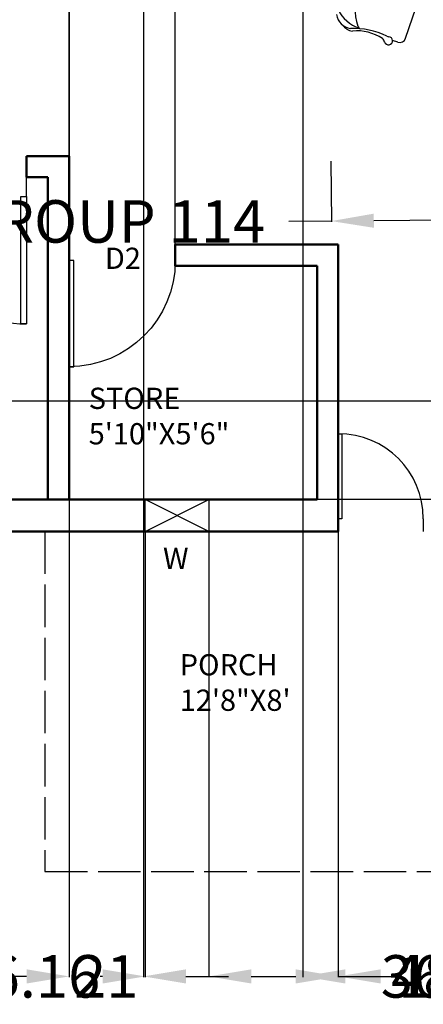
# Model space of a CAD drawing. Units: inches. Extents: x -77 to 516, y -119 to 536.
# Tile 2 of 11: x 150 to 264, y -119 to 159. Entities that reach past the tile are written whole.
import ezdxf

# ---------------------------------------------------------------- set-up
doc = ezdxf.new("R2010")
doc.units = ezdxf.units.IN
doc.header["$MEASUREMENT"] = 0
doc.linetypes.add('ACAD_ISO02W100', pattern=[15, 12, -3])
for name, color, linetype, lineweight in [('A-ANNO-DIMS', 2, 'Continuous', 18), ('A-AREA-IDEN', 170, 'Continuous', 25), ('A-FLOR-PRCH', 40, 'ACAD_ISO02W100', 25), ('doors', 6, 'Continuous', 25), ('furniture', 119, 'Continuous', 18), ('text', 170, 'Continuous', 18), ('walls', 40, 'Continuous', 50), ('windows', 1, 'Continuous', 25)]:
    doc.layers.add(name, color=color, linetype=linetype, lineweight=lineweight)
doc.layers.add('FUR', color=42, linetype='Continuous')
doc.styles.get("Standard").update_dxf_attribs({"font": 'arial.ttf'})
doc.dimstyles.get("Standard").update_dxf_attribs({"dimtxt": 12, "dimasz": 12, "dimexe": 0.18, "dimexo": 0.0625, "dimgap": 0.09, "dimtad": 0, "dimtih": 1, "dimtoh": 1, "dimdec": 1, "dimzin": 0, "dimdsep": 46, "dimlunit": 4, "dimtxsty": 'Standard', "dimcen": 0.09, "dimadec": 0, "dimazin": 0, "dimtfac": 1, "dimtdec": 1, "dimtofl": 0, "dimtmove": 0, "dimatfit": 3, "dimfxl": 1, "dimtolj": 1, "dimtzin": 0, "dimarcsym": 0})

# ---------------------------------------------------------------- blocks, each defined once
blk = doc.blocks.new('*U2')
for p, q in [((0, 0), (0, -6)), ((40, 0), (40, -6))]:
    blk.add_line(p, q)
blk.add_lwpolyline([(0, 0), (0, 40), (1.75, 40), (1.75, 0)], close=True)
blk.add_arc((0, 0), 40, 0, 90)
blk = doc.blocks.new('A$C44A37715')
at = {"layer": 'FUR'}
for p, q in [((3.646, 2.261), (3.416, 1.609)), ((3.734, 2.304), (3.792, 2.283))]:
    blk.add_line(p, q, dxfattribs=at)
for centre, radius, start, end in [((3.837, 2.287), 0.0455, 16.8807, 266.7473), ((3.711, 2.238), 0.0691, 70.5477, 160.5477), ((3.831, 2.187), 0.0553, 63.6571, 86.7473), ((4.239, 3.009), 0.863, 243.6571, 271.4769), ((3.936, 2.308), 0.0553, 187.894, 235.9057), ((4.195, 2.692), 0.519, 235.9057, 274.894), ((3.567, 1.923), 0.642, 303.2315, 17.8639), ((4.125, 2.102), 0.0553, 17.8639, 64.7798), ((4.037, 1.769), 0.394, 24.5429, 71.319), ((4.219, 2.021), 0.155, 33.6596, 82.2991), ((4.228, 1.96), 0.19, 8.9926, 80.0637)]:
    blk.add_arc(centre, radius, start, end, dxfattribs=at)
blk = doc.blocks.new('WIN-18IN')
for p, q in [((18, 0), (0, 9)), ((0, 0), (18, 9))]:
    blk.add_line(p, q)
blk.add_lwpolyline([(0, 9), (18, 9), (18, 0), (0, 0)], close=True)
blk = doc.blocks.new('*D30')
at = {"layer": 'A-ANNO-DIMS', "color": 0, "lineweight": -2, "transparency": 16777216}
for p, q in [((351.13, 120.17), (351.28, 103.03)), ((237.64, 119.18), (237.79, 102.04)), ((339.28, 103.1), (249.78, 102.32)), ((237.78, 102.22), (225.78, 102.12))]:
    blk.add_line(p, q, dxfattribs=at)
at = {"layer": 'A-ANNO-DIMS', "color": 0, "transparency": 16777216}
for points in [[(249.77, 104.32), (249.8, 100.32), (237.78, 102.22)], [(339.27, 105.1), (339.3, 101.1), (351.28, 103.21)]]:
    blk.add_solid(points, dxfattribs=at)
at = {"layer": 'Defpoints', "color": 0, "transparency": 16777216}
for p in [(351.13, 120.23), (237.64, 119.24), (237.78, 102.22)]:
    blk.add_point(p, dxfattribs=at)
at = {"layer": 'A-ANNO-DIMS', "color": 0, "transparency": 16777216, "insert": (140.3, 102.12), "char_height": 12, "attachment_point": 5}
blk.add_mtext('\\A1;SEATING GROUP 114', dxfattribs=at)
blk = doc.blocks.new('*D40')
at = {"layer": 'A-ANNO-DIMS', "color": 0, "lineweight": -2, "transparency": 16777216}
for p, q in [((163.750061, 485.5259), (163.750061, -111.2416)), ((184.750061, 485.5259), (184.750061, -111.2416)), ((151.750061, -111.0616), (139.750061, -111.0616)), ((196.750061, -111.0616), (208.750061, -111.0616))]:
    blk.add_line(p, q, dxfattribs=at)
at = {"layer": 'A-ANNO-DIMS', "color": 0, "transparency": 16777216}
for points in [[(151.750061, -109.0616), (151.750061, -113.0616), (163.750061, -111.0616)], [(196.750061, -109.0616), (196.750061, -113.0616), (184.750061, -111.0616)]]:
    blk.add_solid(points, dxfattribs=at)
at = {"layer": 'Defpoints', "color": 0, "transparency": 16777216}
for p in [(163.750061, 485.5884), (184.750061, 485.5884), (184.750061, -111.0616)]:
    blk.add_point(p, dxfattribs=at)
at = {"layer": 'A-ANNO-DIMS', "color": 0, "transparency": 16777216, "insert": (174.250061, -111.0616), "char_height": 12, "attachment_point": 5}
blk.add_mtext('\\A1;21', dxfattribs=at)
blk = doc.blocks.new('*D41')
at = {"layer": 'A-ANNO-DIMS', "color": 0, "lineweight": -2, "transparency": 16777216}
for p, q in [((229.75, 485.53), (229.75, -111.24)), ((333.59, 485.53), (333.59, -111.24)), ((241.75, -111.06), (257.26, -111.06)), ((321.59, -111.06), (306.08, -111.06))]:
    blk.add_line(p, q, dxfattribs=at)
at = {"layer": 'A-ANNO-DIMS', "color": 0, "transparency": 16777216}
for points in [[(241.75, -109.06), (241.75, -113.06), (229.75, -111.06)], [(321.59, -109.06), (321.59, -113.06), (333.59, -111.06)]]:
    blk.add_solid(points, dxfattribs=at)
at = {"layer": 'Defpoints', "color": 0, "transparency": 16777216}
for p in [(229.75, 485.59), (333.59, 485.59), (333.59, -111.06)]:
    blk.add_point(p, dxfattribs=at)
at = {"layer": 'A-ANNO-DIMS', "color": 0, "transparency": 16777216, "insert": (281.67, -111.06), "char_height": 12, "attachment_point": 5}
blk.add_mtext('\\A1;103.84', dxfattribs=at)
blk = doc.blocks.new('*D45')
at = {"layer": 'A-ANNO-DIMS', "color": 0, "lineweight": -2, "transparency": 16777216}
for p, q in [((-15.9, 51.35), (-15.9, 63.35)), ((-15.9, 63.35), (-3.9, 63.35)), ((364.69, 51.35), (-16.08, 51.35)), ((-15.9, 35.59), (-15.9, 39.35)), ((364.69, 23.59), (-16.08, 23.59))]:
    blk.add_line(p, q, dxfattribs=at)
at = {"layer": 'A-ANNO-DIMS', "color": 0, "transparency": 16777216}
for points in [[(-17.9, 39.35), (-13.9, 39.35), (-15.9, 51.35)], [(-17.9, 35.59), (-13.9, 35.59), (-15.9, 23.59)]]:
    blk.add_solid(points, dxfattribs=at)
at = {"layer": 'Defpoints', "color": 0, "transparency": 16777216}
for p in [(-15.9, 51.35), (364.75, 51.35), (364.75, 23.59)]:
    blk.add_point(p, dxfattribs=at)
at = {"layer": 'A-ANNO-DIMS', "color": 0, "transparency": 16777216, "insert": (16.54, 63.35), "char_height": 12, "attachment_point": 5}
blk.add_mtext('\\A1;27.76', dxfattribs=at)
blk = doc.blocks.new('*D50')
at = {"layer": 'A-ANNO-DIMS', "color": 0, "lineweight": -2, "transparency": 16777216}
for p, q in [((119.05, 14.53), (119.05, -111.24)), ((185.2, 14.53), (185.2, -111.24)), ((131.05, -111.06), (131.76, -111.06)), ((173.2, -111.06), (172.49, -111.06))]:
    blk.add_line(p, q, dxfattribs=at)
at = {"layer": 'A-ANNO-DIMS', "color": 0, "transparency": 16777216}
for points in [[(131.05, -109.06), (131.05, -113.06), (119.05, -111.06)], [(173.2, -109.06), (173.2, -113.06), (185.2, -111.06)]]:
    blk.add_solid(points, dxfattribs=at)
at = {"layer": 'Defpoints', "color": 0, "transparency": 16777216}
for p in [(119.05, 14.59), (185.2, 14.59), (185.2, -111.06)]:
    blk.add_point(p, dxfattribs=at)
at = {"layer": 'A-ANNO-DIMS', "color": 0, "transparency": 16777216, "insert": (152.12, -111.06), "char_height": 12, "attachment_point": 5}
blk.add_mtext('\\A1;66.16', dxfattribs=at)
blk = doc.blocks.new('*D51')
at = {"layer": 'A-ANNO-DIMS', "color": 0, "lineweight": -2, "transparency": 16777216}
for p, q in [((203.2, 14.53), (203.2, -111.24)), ((239.75, 14.53), (239.75, -111.24)), ((215.2, -111.06), (227.75, -111.06)), ((239.75, -111.06), (251.75, -111.06))]:
    blk.add_line(p, q, dxfattribs=at)
at = {"layer": 'A-ANNO-DIMS', "color": 0, "transparency": 16777216}
for points in [[(215.2, -109.06), (215.2, -113.06), (203.2, -111.06)], [(227.75, -109.06), (227.75, -113.06), (239.75, -111.06)]]:
    blk.add_solid(points, dxfattribs=at)
at = {"layer": 'Defpoints', "color": 0, "transparency": 16777216}
for p in [(203.2, 14.59), (239.75, 14.59), (239.75, -111.06)]:
    blk.add_point(p, dxfattribs=at)
at = {"layer": 'A-ANNO-DIMS', "color": 0, "transparency": 16777216, "insert": (276.74, -111.06), "char_height": 12, "attachment_point": 5}
blk.add_mtext('\\A1;36.546', dxfattribs=at)
blk = doc.blocks.new('*D52')
at = {"layer": 'A-ANNO-DIMS', "color": 0, "lineweight": -2, "transparency": 16777216}
for p, q in [((239.75, 14.53), (239.75, -111.24)), ((287.75, 14.53), (287.75, -111.24)), ((251.75, -111.06), (254.81, -111.06)), ((275.75, -111.06), (272.69, -111.06))]:
    blk.add_line(p, q, dxfattribs=at)
at = {"layer": 'A-ANNO-DIMS', "color": 0, "transparency": 16777216}
for points in [[(251.75, -109.06), (251.75, -113.06), (239.75, -111.06)], [(275.75, -109.06), (275.75, -113.06), (287.75, -111.06)]]:
    blk.add_solid(points, dxfattribs=at)
at = {"layer": 'Defpoints', "color": 0, "transparency": 16777216}
for p in [(239.75, 14.59), (287.75, 14.59), (287.75, -111.06)]:
    blk.add_point(p, dxfattribs=at)
at = {"layer": 'A-ANNO-DIMS', "color": 0, "transparency": 16777216, "insert": (263.75, -111.06), "char_height": 12, "attachment_point": 5}
blk.add_mtext('\\A1;48', dxfattribs=at)
blk = doc.blocks.new('*D53')
at = {"layer": 'A-ANNO-DIMS', "color": 0, "lineweight": -2, "transparency": 16777216}
for p, q in [((163.75, 95.65), (163.75, 525.13)), ((175.75, 524.95), (181.75, 524.95)), ((193.75, 95.65), (193.75, 525.13)), ((193.75, 524.95), (205.75, 524.95))]:
    blk.add_line(p, q, dxfattribs=at)
at = {"layer": 'A-ANNO-DIMS', "color": 0, "transparency": 16777216}
for points in [[(175.75, 526.95), (175.75, 522.95), (163.75, 524.95)], [(181.75, 526.95), (181.75, 522.95), (193.75, 524.95)]]:
    blk.add_solid(points, dxfattribs=at)
at = {"layer": 'Defpoints', "color": 0, "transparency": 16777216}
for p in [(193.75, 524.95), (163.75, 95.59), (193.75, 95.59)]:
    blk.add_point(p, dxfattribs=at)
at = {"layer": 'A-ANNO-DIMS', "color": 0, "transparency": 16777216, "insert": (214.41, 524.95), "char_height": 12, "attachment_point": 5}
blk.add_mtext('\\A1;30', dxfattribs=at)

msp = doc.modelspace()

# ---------------------------------------------------------------- linework, layer by layer
at = {"layer": 'A-FLOR-PRCH'}
msp.add_line((156.9336, 14.5884), (156.9336, -81.4116), dxfattribs=at)
msp.add_lwpolyline([(156.9336, -81.4116), (308.9336, -81.4116)], dxfattribs=at)
at = {"layer": 'walls'}
for p, q in [((151.7501, 120.5884), (151.7501, 114.5884)), ((151.7501, 120.5884), (163.7501, 120.5884)), ((163.7501, 120.5884), (163.7501, 23.5884)), ((151.7501, 114.5884), (157.7501, 114.5884)), ((157.7501, 114.5884), (157.7501, 23.5884)), ((193.7501, 95.5884), (239.7501, 95.5884)), ((193.7501, 95.5884), (193.7501, 89.5884)), ((193.7501, 95.5884), (239.7501, 95.5884)), ((239.7501, 95.5884), (239.7501, 14.5884)), ((193.7501, 89.5884), (233.7501, 89.5884)), ((193.7501, 89.5884), (233.7501, 89.5884)), ((233.7501, 89.5884), (233.7501, 23.5884)), ((22.7501, 23.5884), (233.7501, 23.5884))]:
    msp.add_line(p, q, dxfattribs=at)
msp.add_lwpolyline([(373.7501, 131.5884), (373.7501, 494.5884), (13.7501, 494.5884), (13.7501, 14.5884), (239.7501, 14.5884)], dxfattribs=at)

# ---------------------------------------------------------------- block references
at = {"layer": 'doors', "rotation": 180}
for p, xscale, yscale, zscale in [((151.7501, 109.1884), 0.9000000000000007, 0.9000000000000007, 0.9000000000000007), ((163.7501, 91.0884), -0.7500000000000016, 0.7500000000000016, 0.7500000000000016)]:
    msp.add_blockref('*U2', p, dxfattribs=dict(at, xscale=xscale, yscale=yscale, zscale=zscale))
at = {"layer": 'doors', "xscale": 0.6000000000000032, "yscale": 0.6000000000000032, "zscale": 0.6000000000000032}
msp.add_blockref('*U2', (239.7501, 18.1884), dxfattribs=at)
at = {"layer": 'furniture', "xscale": 25.25763254760833, "yscale": 25.25763254760833, "zscale": 25.25763254760833, "rotation": 180.4978074292498}
msp.add_blockref('A$C44A37715', (350.3392, 211.7368), dxfattribs=at)
at = {"layer": 'windows'}
msp.add_blockref('WIN-18IN', (185.2037, 14.588), dxfattribs=at)

# ---------------------------------------------------------------- texts
at = {"layer": 'A-AREA-IDEN', "char_height": 6, "attachment_point": 1}
for s, insert in [('STORE\\P5\'10"X5\'6"', (169.2996, 55.1737)), ('PORCH\\P12\'8"X8\'', (194.9896, -20.0671))]:
    msp.add_mtext_dynamic_manual_height_columns(s, width=105.041962, gutter_width=1, heights=[0], dxfattribs=dict(at, insert=insert))
at = {"layer": 'text', "char_height": 6, "attachment_point": 1}
for s, insert in [('D2', (173.8739, 94.7124)), ('W', (190.2874, 9.9642))]:
    msp.add_mtext_dynamic_manual_height_columns(s, width=105.041962, gutter_width=1, heights=[0], dxfattribs=dict(at, insert=insert))

# ---------------------------------------------------------------- dimensions: what is measured, and where the dimension line sits
at = {"layer": 'A-ANNO-DIMS'}
for base, p1, p2, override, picture, middle in [((193.7501, 524.9457), (163.7501, 95.5884), (193.7501, 95.5884), {"dimdec": 0, "dimlfac": 1, "dimrnd": 0, "dimzin": 0, "dimdsep": 46, "dimlunit": 2}, '*D53', (214.4103, 524.9457)), ((184.7501, -111.0616), (163.7501, 485.5884), (184.7501, 485.5884), {"dimdec": 0, "dimlfac": 1, "dimrnd": 0, "dimzin": 0, "dimdsep": 46, "dimlunit": 2}, '*D40', (174.2501, -111.0616)), ((333.5885, -111.0616), (229.7501, 485.5884), (333.5885, 485.5884), {"dimdec": 2, "dimlfac": 1, "dimrnd": 0, "dimzin": 0, "dimdsep": 46, "dimlunit": 2}, '*D41', (281.6693, -111.0616)), ((185.2037, -111.0616), (119.0451, 14.5884), (185.2037, 14.5884), {"dimdec": 2, "dimlfac": 1, "dimrnd": 0, "dimzin": 0, "dimdsep": 46, "dimlunit": 2}, '*D50', (152.1244, -111.0616)), ((239.7501, -111.0616), (203.2037, 14.5884), (239.7501, 14.5884), {"dimdec": 3, "dimlfac": 1, "dimrnd": 0, "dimzin": 0, "dimdsep": 46, "dimlunit": 2}, '*D51', (276.7405, -111.0616)), ((287.7501, -111.0616), (239.7501, 14.5884), (287.7501, 14.5884), {"dimdec": 0, "dimlfac": 1, "dimrnd": 0, "dimzin": 0, "dimdsep": 46, "dimlunit": 2}, '*D52', (263.7501, -111.0616))]:
    dim = msp.add_linear_dim(base=base, p1=p1, p2=p2, dimstyle='Standard', override=override, dxfattribs=at)
    dim.commit()
    dim.dimension.update_dxf_attribs({"geometry": picture, "text_midpoint": middle})
dim = msp.add_linear_dim(base=(237.7836, 102.22), p1=(351.1342, 120.231), p2=(237.6357, 119.2448), angle=180.497807, text='SEATING GROUP <>', dimstyle='Standard', override={"dimdec": 0, "dimlfac": 1, "dimrnd": 0, "dimzin": 0, "dimdsep": 46, "dimlunit": 2}, dxfattribs=at)
dim.commit()
dim.dimension.update_dxf_attribs({"geometry": '*D30', "text_midpoint": (140.3025, 102.1158)})
dim = msp.add_linear_dim(base=(-15.8999, 51.3473), p1=(364.7501, 23.5884), p2=(364.7501, 51.3473), angle=90, dimstyle='Standard', override={"dimdec": 2, "dimlfac": 1, "dimrnd": 0, "dimzin": 0, "dimdsep": 46, "dimlunit": 2}, dxfattribs=at)
dim.commit()
dim.dimension.update_dxf_attribs({"geometry": '*D45', "text_midpoint": (16.5352, 63.3473)})

doc.saveas('drawing.dxf')
